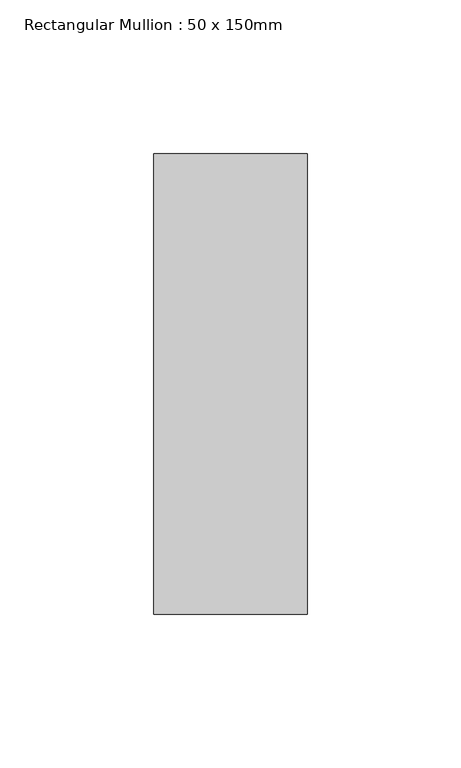
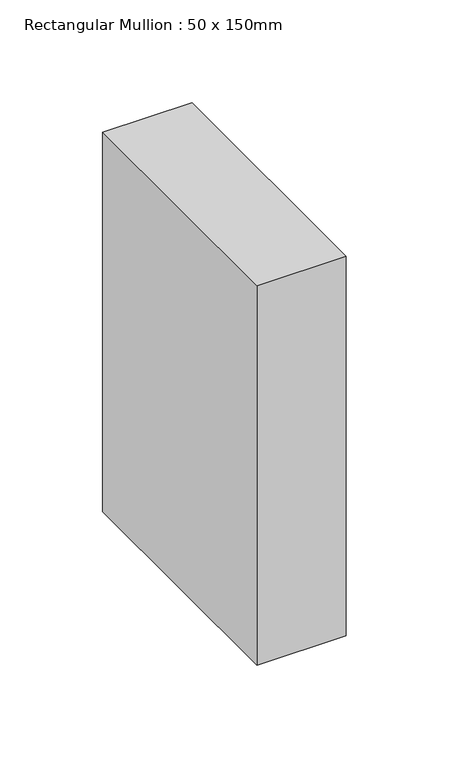
"""IFC4 building model written with IfcOpenShell, lengths in millimetres: member geometry, Rectangular Mullion : 50 x 150mm."""

from ifc_helpers import new_model, si_unit, frame, origin, place, context, project, spatial, polyline, outline, extrude, source, transform, mapped, element, save


def rectangular_mullion_50_x_150mm_ef1c4831(model_context):
    return source(origin(), model_context, "Body", "SweptSolid", [
        extrude(outline(polyline([(0.0, 75.0), (0.0, -75.0), (-50.0, -75.0), (-50.0, 75.0), (0.0, 75.0)])), frame((0.0, 0.0, -225.0), z_axis=(0.0, 0.0, 1.0), x_axis=(1.0, 0.0, 0.0)), (0.0, 0.0, 1.0), 225.0),
    ])


if __name__ == "__main__":
    model = new_model("IFC4")
    model_context = context("Model", 3, world=origin())
    ifc_project = project(units=[si_unit("LENGTHUNIT", "METRE", prefix="MILLI")], contexts=[model_context])
    site = spatial("IfcSite", under=ifc_project)
    building = spatial("IfcBuilding", under=site)
    placement = place(None, origin())
    rectangular_mullion_50_x_150mm_shape = rectangular_mullion_50_x_150mm_ef1c4831(model_context)
    element("IfcMember", 1, ObjectType="Rectangular Mullion : 50 x 150mm", at=placement, inside=building, context=model_context, shape_type="MappedRepresentation", body=[
        mapped(rectangular_mullion_50_x_150mm_shape, transform((0.0, 0.0, 0.0), x_axis=(1.0, 0.0, 0.0), y_axis=(0.0, 1.0, 0.0), z_axis=(0.0, 0.0, 1.0))),
    ])
    save(model, "model.ifc")

# Revit data of these elements
# Type "Rectangular Mullion : 50 x 150mm"
#   built-in parameter 1007304 = 0.492126 (stored number, unit not read)
#   built-in parameter 1007301 = 0.082021 (stored number, unit not read)
#   built-in parameter 1007300 = 0.082021 (stored number, unit not read)
# Element 1 (IfcMember, "Rectangular Mullion : 50 x 150mm")
#   Materials on its faces: "Aluminium"
# Materials
#   "Aluminium": class "Metal", colour RGB 247 247 247, transparency 0, Description = "Aluminium 6061", Cost = 0
